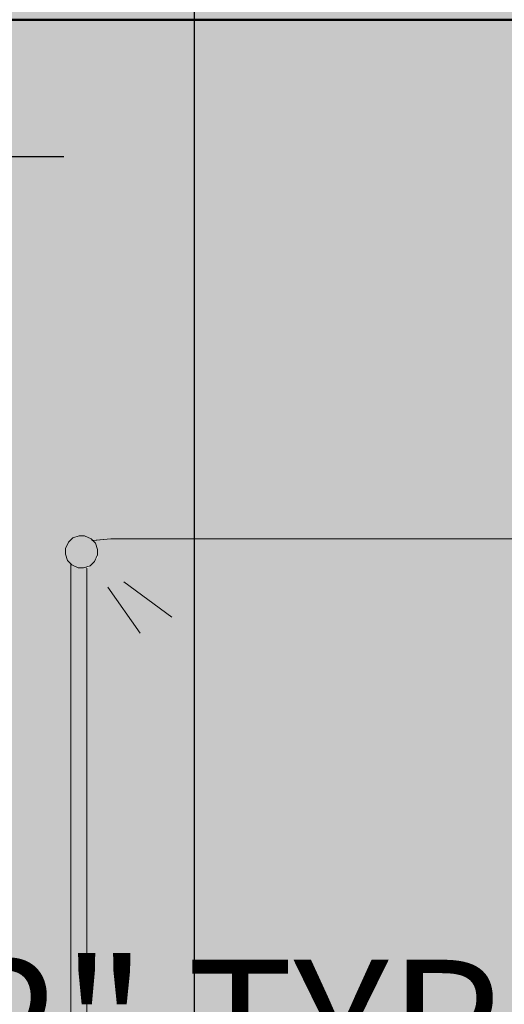
# Model space of a CAD drawing. Units: inches. Extents: x 528 to 2620, y -1066 to 798.
# Tile 29 of 41: x 1157 to 1180, y 665 to 710. Entities that reach past the tile are written whole.
import ezdxf

# ---------------------------------------------------------------- set-up
doc = ezdxf.new("R2010")
doc.units = ezdxf.units.IN
doc.header["$MEASUREMENT"] = 0
for name, color, linetype, lineweight in [('A-ANNO-DIMS', 2, 'Continuous', 18), ('A-FURN', 30, 'Continuous', 18), ('A-WALL', 7, 'Continuous', 50), ('A-WALL-PATT', 8, 'Continuous', 13)]:
    doc.layers.add(name, color=color, linetype=linetype, lineweight=lineweight)
doc.styles.get("Standard").update_dxf_attribs({"font": 'arial.ttf'})
doc.dimstyles.get("Standard").update_dxf_attribs({"dimtxt": 6, "dimasz": 2, "dimexe": 0.18, "dimexo": 0.0625, "dimgap": 0.09, "dimtad": 0, "dimtih": 1, "dimtoh": 1, "dimdec": 1, "dimzin": 0, "dimdsep": 46, "dimlunit": 3, "dimtxsty": 'Standard', "dimblk": 'ARCHTICK', "dimcen": 0.09, "dimadec": 0, "dimazin": 0, "dimtfac": 1, "dimtdec": 1, "dimtofl": 0, "dimtmove": 0, "dimatfit": 3, "dimfxl": 1, "dimtolj": 1, "dimtzin": 0, "dimarcsym": 0})

# ---------------------------------------------------------------- blocks, each defined once
blk = doc.blocks.new('d-bed-3')
at = {"color": 0, "linetype": 'ByBlock'}
for p, q in [((0.7857, -2.0939), (0.7857, -0.0297)), ((0.7857, -0.032), (0.7857, -2.0939)), ((0.8741, -2.0673), (0.9464, -1.9691)), ((0.8851, -2.1005), (0.9795, -2.0342)), ((0.7888, -2.1317), (0.7857, -2.0939)), ((0.7857, -2.0939), (0.7887, -2.1303)), ((0.7948, -2.1259), (0.8078, -2.1215)), ((0.8078, -2.1215), (0.8188, -2.1215)), ((0.8188, -2.1215), (0.8319, -2.1281)), ((0.7797, -2.148), (0.7857, -2.1347)), ((0.7797, -2.148), (0.7857, -2.1347)), ((0.7857, -2.1347), (0.7948, -2.1259)), ((0.7857, -2.1347), (0.7888, -2.1317)), ((0.8319, -2.1281), (0.8409, -2.1369)), ((0.8409, -2.1369), (0.845, -2.1502)), ((2.7264, -2.1436), (0.845, -2.1436)), ((0.7797, -2.159), (0.7797, -2.148)), ((0.7797, -2.148), (0.7797, -2.159)), ((0.7837, -2.1723), (0.7797, -2.159)), ((0.7837, -2.1723), (0.7797, -2.159)), ((0.845, -2.1612), (0.8389, -2.1745)), ((0.845, -2.1502), (0.845, -2.1612)), ((0.7927, -2.1811), (0.7837, -2.1723)), ((0.7927, -2.1811), (0.7837, -2.1723)), ((0.8058, -2.1877), (0.7927, -2.1811)), ((0.8058, -2.1877), (0.7927, -2.1811)), ((0.8299, -2.1833), (0.8168, -2.1877)), ((0.8299, -2.1833), (0.8168, -2.1877)), ((0.8389, -2.1745), (0.8299, -2.1833)), ((0.8367, -2.1767), (0.8299, -2.1833)), ((2.7327, -2.1767), (0.8367, -2.1767)), ((0.8389, -2.1767), (2.7305, -2.1767)), ((0.8168, -2.1877), (0.8058, -2.1877)), ((0.8168, -2.1877), (0.8058, -2.1877))]:
    blk.add_line(p, q, dxfattribs=at)
blk = doc.blocks.new('_ArchTick')
at = {"color": 0, "linetype": 'ByBlock', "const_width": 0.15}
blk.add_lwpolyline([(-0.5, -0.5), (0.5, 0.5)], dxfattribs=at)
blk = doc.blocks.new('*D42')
at = {"layer": 'A-ANNO-DIMS', "color": 0, "lineweight": -2, "transparency": 16777216}
for p, q in [((1159.521, 703.64), (1147.464, 703.64)), ((1147.644, 703.64), (1147.644, 667.032)), ((1147.644, 624.039), (1147.644, 660.647)), ((1159.521, 624.039), (1147.464, 624.039))]:
    blk.add_line(p, q, dxfattribs=at)
at = {"layer": 'Defpoints', "color": 0, "transparency": 16777216}
for p in [(1159.584, 703.64), (1147.644, 624.039), (1159.584, 624.039)]:
    blk.add_point(p, dxfattribs=at)
at = {"layer": 'A-ANNO-DIMS', "color": 0, "lineweight": -2, "transparency": 16777216, "xscale": 2, "yscale": 2, "zscale": 2}
for p, rotation in [((1147.644, 703.64), 90), ((1147.644, 624.039), 270)]:
    blk.add_blockref('_ArchTick', p, dxfattribs=dict(at, rotation=rotation))
at = {"layer": 'A-ANNO-DIMS', "color": 0, "transparency": 16777216, "insert": (1147.644, 663.839), "char_height": 6, "attachment_point": 5}
blk.add_mtext('\\A1;BED 6\'-7 1/2" TYP.', dxfattribs=at)
blk = doc.blocks.new('*D58')
at = {"layer": 'A-ANNO-DIMS', "color": 0, "lineweight": -2, "transparency": 16777216}
for p, q in [((1165.496, 577.985), (1165.496, 751.102)), ((1165.496, 750.922), (1177.395, 750.922)), ((1205.418, 750.922), (1193.52, 750.922)), ((1205.418, 577.985), (1205.418, 751.102))]:
    blk.add_line(p, q, dxfattribs=at)
at = {"layer": 'Defpoints', "color": 0, "transparency": 16777216}
for p in [(1205.418, 750.922), (1165.496, 577.922), (1205.418, 577.922)]:
    blk.add_point(p, dxfattribs=at)
at = {"layer": 'A-ANNO-DIMS', "color": 0, "lineweight": -2, "transparency": 16777216, "xscale": 2, "yscale": 2, "zscale": 2, "rotation": 180}
blk.add_blockref('_ArchTick', (1165.496, 750.922), dxfattribs=at)
at = {"layer": 'A-ANNO-DIMS', "color": 0, "lineweight": -2, "transparency": 16777216, "xscale": 2, "yscale": 2, "zscale": 2}
blk.add_blockref('_ArchTick', (1205.418, 750.922), dxfattribs=at)
at = {"layer": 'A-ANNO-DIMS', "color": 0, "transparency": 16777216, "insert": (1185.457, 750.922), "char_height": 6, "attachment_point": 5}
blk.add_mtext('\\A1;3\'-4"', dxfattribs=at)

msp = doc.modelspace()

# ---------------------------------------------------------------- hatches: boundary and pattern name
at = {"layer": 'A-WALL-PATT', "transparency": 33554521}
h = msp.add_hatch(color=256, dxfattribs=at)
h.dxf.hatch_style = 1
h.paths.add_polyline_path([(1065.996, 709.922), (1114.496, 709.922), (1114.496, 718.922), (1056.996, 718.922), (1056.996, 667.922), (1065.996, 667.922)])
h.paths.add_polyline_path([(1227.496, 718.922), (1162.496, 718.922), (1162.496, 709.922), (1210.996, 709.922), (1210.996, 577.922), (1205.418, 577.922), (1205.496, 573.422), (1210.996, 573.422), (1210.996, 567.422), (1215.496, 567.422), (1215.496, 669.422), (1267.996, 669.422), (1267.996, 675.922), (1263.496, 675.922), (1263.496, 673.922), (1215.496, 673.922), (1215.496, 709.922), (1227.496, 709.922)])
h.paths.add_polyline_path([(1344.996, 718.922), (1315.996, 718.922), (1315.996, 709.922), (1335.996, 709.922), (1335.996, 641.672), (1344.996, 641.672)])
h.paths.add_polyline_path([(1065.996, 619.922), (1056.996, 619.922), (1056.996, 561.422), (1065.996, 561.422), (1065.996, 573.422), (1160.996, 573.422), (1160.996, 569.422), (1165.496, 569.422), (1165.496, 577.922), (1065.996, 577.922)])
h.paths.add_polyline_path([(1215.996, 391.422), (1215.996, 400.422), (1206.996, 400.422), (1200.996, 400.422), (1200.996, 397.422), (1200.996, 391.422), (1206.996, 391.422), (1206.996, 268.922), (1251.996, 268.922), (1251.996, 277.922), (1215.996, 277.922), (1215.996, 359.767)])
h.paths.add_polyline_path([(1344.996, 395.922), (1335.996, 395.922), (1287.996, 395.922), (1287.996, 391.422), (1335.996, 391.422), (1335.996, 277.922), (1299.996, 277.922), (1299.996, 268.922), (1344.996, 268.922)])
h.paths.add_polyline_path([(1344.996, 593.672), (1335.996, 593.672), (1335.996, 525.422), (1215.496, 525.422), (1215.496, 527.172), (1210.996, 527.172), (1210.996, 520.922), (1335.996, 520.922), (1335.996, 443.922), (1344.996, 443.922)])
h.paths.add_polyline_path([(1065.996, 520.922), (1165.496, 520.922), (1165.496, 545.422), (1160.996, 545.422), (1160.996, 525.422), (1065.996, 525.422), (1065.996, 537.422), (1056.996, 537.422), (1056.996, 484.672), (1065.996, 484.672)])
h.paths.add_polyline_path([(1065.996, 436.672), (1056.996, 436.672), (1056.996, 391.422), (1085.496, 391.422), (1085.496, 400.422), (1065.996, 400.422)])
h.paths.add_polyline_path([(1152.996, 397.422), (1152.996, 400.422), (1133.496, 400.422), (1133.496, 391.422), (1152.996, 391.422)])
at = {"layer": 'A-WALL-PATT', "transparency": 33554681}
h = msp.add_hatch(color=256, dxfattribs=at)
h.dxf.hatch_style = 1
h.paths.add_polyline_path([(1061.996, 665.922), (1060.996, 665.922), (1060.996, 621.922), (1061.996, 621.922)])
h.paths.add_polyline_path([(1065.996, 667.922), (1056.996, 667.922), (1056.996, 665.922), (1065.996, 665.922)])
h.paths.add_polyline_path([(1065.996, 621.922), (1056.996, 621.922), (1056.996, 619.922), (1065.996, 619.922)])
h.paths.add_polyline_path([(1160.496, 714.922), (1116.496, 714.922), (1116.496, 713.922), (1160.496, 713.922)])
h.paths.add_polyline_path([(1162.496, 718.922), (1160.496, 718.922), (1160.496, 709.922), (1162.496, 709.922)])
h.paths.add_polyline_path([(1116.496, 718.922), (1114.496, 718.922), (1114.496, 709.922), (1116.496, 709.922)])
h.paths.add_polyline_path([(1251.496, 714.922), (1227.496, 714.922), (1227.496, 713.922), (1251.496, 713.922)])
h.paths.add_polyline_path([(1313.996, 714.922), (1269.996, 714.922), (1269.996, 713.922), (1313.996, 713.922)])
h.paths.add_polyline_path([(1315.996, 718.922), (1313.996, 718.922), (1313.996, 709.922), (1315.996, 709.922)])
h.paths.add_polyline_path([(1269.996, 718.922), (1267.996, 718.922), (1267.996, 709.922), (1269.996, 709.922)])
h.paths.add_polyline_path([(1087.496, 400.422), (1085.496, 400.422), (1085.496, 391.422), (1087.496, 391.422)])
h.paths.add_polyline_path([(1131.496, 396.422), (1087.496, 396.422), (1087.496, 395.422), (1131.496, 395.422)])
h.paths.add_polyline_path([(1133.496, 400.422), (1131.496, 400.422), (1131.496, 391.422), (1133.496, 391.422)])
h.paths.add_polyline_path([(1065.996, 438.672), (1056.996, 438.672), (1056.996, 436.672), (1065.996, 436.672)])
h.paths.add_polyline_path([(1065.996, 484.672), (1056.996, 484.672), (1056.996, 482.672), (1065.996, 482.672)])
h.paths.add_polyline_path([(1061.996, 482.672), (1060.996, 482.672), (1060.996, 438.672), (1061.996, 438.672)])
h = msp.add_hatch(color=256, dxfattribs=at)
h.dxf.hatch_style = 1
h.paths.add_polyline_path([(1065.996, 665.922), (1061.996, 665.922), (1061.996, 621.922), (1065.996, 621.922)])
h.paths.add_polyline_path([(1060.996, 665.922), (1056.996, 665.922), (1056.996, 621.922), (1060.996, 621.922)])
h.paths.add_polyline_path([(1160.496, 713.922), (1116.496, 713.922), (1116.496, 709.922), (1160.496, 709.922)])
h.paths.add_polyline_path([(1160.496, 718.922), (1116.496, 718.922), (1116.496, 714.922), (1160.496, 714.922)])
h.paths.add_polyline_path([(1251.496, 713.922), (1227.496, 713.922), (1227.496, 709.922), (1251.496, 709.922)])
h.paths.add_polyline_path([(1251.496, 718.922), (1227.496, 718.922), (1227.496, 714.922), (1251.496, 714.922)])
h.paths.add_polyline_path([(1313.996, 713.922), (1269.996, 713.922), (1269.996, 709.922), (1313.996, 709.922)])
h.paths.add_polyline_path([(1313.996, 718.922), (1269.996, 718.922), (1269.996, 714.922), (1313.996, 714.922)])
h.paths.add_polyline_path([(1344.996, 639.672), (1340.996, 639.672), (1340.996, 595.672), (1344.996, 595.672)])
h.paths.add_polyline_path([(1339.996, 639.672), (1335.996, 639.672), (1335.996, 595.672), (1339.996, 595.672)])
h.paths.add_polyline_path([(1344.996, 441.922), (1340.996, 441.922), (1340.996, 397.922), (1344.996, 397.922)])
h.paths.add_polyline_path([(1339.996, 441.922), (1335.996, 441.922), (1335.996, 397.922), (1339.996, 397.922)])
h.paths.add_polyline_path([(1297.996, 272.922), (1253.996, 272.922), (1253.996, 268.922), (1297.996, 268.922)])
h.paths.add_polyline_path([(1297.996, 277.922), (1253.996, 277.922), (1253.996, 273.922), (1297.996, 273.922)])
h.paths.add_polyline_path([(1131.496, 395.422), (1087.496, 395.422), (1087.496, 391.422), (1131.496, 391.422)])
h.paths.add_polyline_path([(1131.496, 400.422), (1087.496, 400.422), (1087.496, 396.422), (1131.496, 396.422)])
h.paths.add_polyline_path([(1065.996, 482.672), (1061.996, 482.672), (1061.996, 438.672), (1065.996, 438.672)])
h.paths.add_polyline_path([(1060.996, 482.672), (1056.996, 482.672), (1056.996, 438.672), (1060.996, 438.672)])
h.paths.add_polyline_path([(1065.996, 561.422), (1061.996, 561.422), (1061.996, 537.422), (1065.996, 537.422)])
h.paths.add_polyline_path([(1060.996, 561.422), (1056.996, 561.422), (1056.996, 537.422), (1060.996, 537.422)])
at = {"layer": 'A-WALL-PATT', "transparency": 33554536}
h = msp.add_hatch(color=256, dxfattribs=at)
h.dxf.hatch_style = 1
h.paths.add_polyline_path([(1335.996, 709.922), (1267.996, 709.922), (1267.996, 699.922), (1266.746, 699.922), (1266.746, 675.922), (1267.996, 675.922), (1267.996, 669.422), (1215.496, 669.422), (1215.496, 567.172), (1216.996, 567.172), (1256.996, 567.172), (1256.996, 565.422), (1256.958, 565.422, -0.401453), (1216.996, 527.172), (1215.496, 527.172), (1215.496, 525.422), (1335.996, 525.422)], flags=17)
h.paths.add_polyline_path([(1285.032, 635.927), (1285.229, 636.128), (1285.672, 636.263), (1286.206, 636.02), (1286.976, 636.084), (1332.983, 636.084), (1333.363, 636.222), (1333.82, 636.084), (1334.115, 635.714), (1334.115, 635.3), (1333.907, 634.86), (1333.82, 634.827), (1333.82, 592.738), (1333.967, 592.604), (1334.115, 592.291), (1334.115, 591.877), (1333.82, 591.507), (1333.363, 591.369), (1332.983, 591.507), (1332.638, 591.789), (1332.638, 591.507), (1286.976, 591.507), (1286.173, 591.672), (1286.066, 591.574), (1285.681, 591.37), (1285.229, 591.507), (1285.032, 591.709), (1284.834, 592.098), (1284.983, 592.537), (1285.13, 592.688), (1285.13, 634.948), (1284.983, 635.099), (1284.834, 635.537)], flags=16)
h.paths.add_polyline_path([(1285.032, 635.927), (1285.229, 636.128), (1285.672, 636.263), (1286.206, 636.02), (1286.976, 636.084), (1332.983, 636.084), (1333.363, 636.222), (1333.82, 636.084), (1334.115, 635.714), (1334.115, 635.3), (1333.967, 634.987), (1333.82, 634.853), (1333.82, 592.738), (1333.967, 592.604), (1334.115, 592.291), (1334.115, 591.877), (1333.82, 591.507), (1333.363, 591.369), (1332.983, 591.507), (1332.638, 591.789), (1332.638, 592.246), (1332.638, 635.345), (1332.638, 635.802), (1332.983, 636.084), (1312.232, 636.084), (1311.1, 635.479), (1310.632, 635.479), (1310.435, 635.233), (1309.943, 635.099), (1309.696, 634.987), (1309.056, 634.763), (1308.712, 634.607), (1308.318, 634.607), (1307.752, 634.36), (1307.112, 634.271), (1307.013, 634.114), (1306.767, 634.025), (1307.255, 633.283), (1306.866, 633.04), (1306.767, 632.884), (1306.373, 632.637), (1306.029, 632.548), (1305.536, 632.414), (1315.472, 618.494), (1316.321, 619.388), (1312.773, 622.858), (1319.616, 630.109), (1320.067, 629.676), (1320.109, 629.997), (1320.281, 630.601), (1320.527, 631.183), (1320.527, 632.011), (1320.256, 632.548), (1320.109, 633.13), (1320.06, 633.734), (1320.626, 634.025), (1321.216, 634.159), (1321.856, 634.114), (1322.447, 633.913), (1322.989, 633.622), (1324.096, 633.622), (1324.638, 633.913), (1325.229, 634.07), (1325.869, 634.07), (1326.435, 633.913), (1326.976, 633.622), (1328.355, 633.622), (1328.896, 633.913), (1329.487, 634.114), (1330.103, 634.159), (1330.693, 634.025), (1331.284, 633.734), (1331.235, 633.13), (1331.087, 632.548), (1330.792, 632.011), (1330.792, 631.183), (1331.038, 630.601), (1331.235, 629.997), (1331.284, 629.415), (1331.186, 628.788), (1331.038, 628.184), (1330.792, 627.602), (1330.792, 626.774), (1331.038, 626.193), (1331.235, 625.588), (1331.284, 625.007), (1331.186, 624.38), (1331.038, 623.776), (1330.792, 623.239), (1330.792, 622.366), (1331.038, 621.829), (1331.235, 621.247), (1331.284, 620.598), (1331.186, 619.972), (1331.038, 619.367), (1330.792, 618.83), (1330.792, 617.958), (1331.087, 617.421), (1331.235, 616.884), (1331.284, 616.235), (1331.284, 615.518), (1330.693, 615.272), (1330.103, 615.116), (1329.487, 615.116), (1328.896, 615.317), (1328.355, 615.653), (1326.976, 615.653), (1326.435, 615.317), (1325.869, 615.16), (1325.229, 615.16), (1324.638, 615.317), (1324.096, 615.653), (1323.242, 615.653), (1324.933, 614.042), (1322.978, 611.983), (1324.096, 611.983), (1324.638, 612.274), (1325.278, 612.43), (1325.869, 612.43), (1326.484, 612.274), (1327.026, 611.983), (1328.355, 611.983), (1328.896, 612.274), (1329.487, 612.475), (1330.103, 612.52), (1330.743, 612.386), (1331.284, 612.072), (1331.284, 611.356), (1331.284, 610.752), (1331.087, 610.17), (1330.792, 609.633), (1330.792, 608.805), (1331.087, 608.223), (1331.235, 607.619), (1331.284, 606.993), (1331.235, 606.411), (1331.087, 605.807), (1330.792, 605.225), (1330.792, 604.397), (1331.087, 603.815), (1331.235, 603.211), (1331.284, 602.629), (1331.235, 602.002), (1331.087, 601.398), (1330.792, 600.861), (1330.792, 599.988), (1331.087, 599.451), (1331.235, 598.87), (1331.284, 598.221), (1331.235, 597.594), (1331.087, 596.99), (1330.792, 596.453), (1330.792, 595.58), (1331.087, 595.043), (1331.284, 594.506), (1331.284, 593.857), (1330.743, 593.611), (1330.103, 593.477), (1329.487, 593.477), (1328.896, 593.678), (1328.355, 594.014), (1327.026, 594.014), (1326.484, 593.678), (1325.869, 593.521), (1325.278, 593.521), (1324.638, 593.678), (1324.096, 594.014), (1323.038, 594.014), (1322.496, 593.678), (1321.906, 593.477), (1321.266, 593.477), (1320.626, 593.611), (1320.109, 593.857), (1320.109, 594.506), (1320.281, 595.043), (1320.576, 595.58), (1320.576, 596.453), (1320.281, 596.99), (1320.158, 597.594), (1320.104, 598.015), (1319.616, 597.549), (1315.659, 601.729), (1312.232, 591.574), (1311.74, 591.664), (1311.592, 591.91), (1310.78, 592.402), (1309.549, 592.895), (1308.958, 592.895), (1308.712, 593.029), (1308.564, 593.141), (1307.752, 593.521), (1306.767, 593.611), (1307.248, 594.356), (1306.866, 594.595), (1306.373, 594.842), (1306.029, 595.088), (1305.536, 595.244), (1315.465, 609.354), (1310.927, 613.706), (1315.472, 618.494), (1305.536, 632.414), (1306.029, 632.548), (1306.373, 632.637), (1306.767, 632.884), (1306.866, 633.04), (1307.255, 633.283), (1306.767, 634.025), (1307.013, 634.114), (1307.112, 634.271), (1307.752, 634.36), (1308.318, 634.607), (1308.712, 634.607), (1309.056, 634.763), (1309.696, 634.987), (1309.943, 635.099), (1310.435, 635.233), (1310.632, 635.479), (1311.1, 635.479), (1312.232, 636.084), (1286.976, 636.084), (1286.216, 636.021), (1286.411, 635.444), (1286.213, 635.054), (1286.016, 634.853), (1285.869, 634.808), (1285.869, 592.839), (1286.153, 592.731), (1286.41, 592.188), (1286.231, 591.66), (1286.173, 591.672), (1286.066, 591.574), (1285.681, 591.37), (1285.229, 591.507), (1285.032, 591.709), (1284.834, 592.098), (1284.983, 592.537), (1285.13, 592.688), (1285.13, 634.948), (1284.983, 635.099), (1284.834, 635.537)], flags=0)
h.paths.add_polyline_path([(1322.501, 653.596), (1333.646, 653.596), (1333.646, 637.994), (1322.501, 637.994)], flags=16)
h.paths.add_polyline_path([(1323.616, 652.482), (1332.531, 652.482), (1332.531, 639.108), (1323.616, 639.108)], flags=0)
edge = h.paths.add_edge_path(flags=0)
edge.add_ellipse((1328.073, 645.795), major_axis=(2.245, 2.245), ratio=1, start_angle=405, end_angle=495, ccw=False)
edge.add_ellipse((1328.073, 645.795), major_axis=(2.245, 2.245), ratio=1, start_angle=675, end_angle=765, ccw=False)
edge.add_ellipse((1328.073, 645.795), major_axis=(2.245, 2.245), ratio=1, start_angle=585, end_angle=675, ccw=False)
edge.add_ellipse((1328.073, 645.795), major_axis=(2.245, 2.245), ratio=1, start_angle=495, end_angle=585, ccw=False)
h.paths.add_polyline_path([(1320.576, 628.386), (1320.33, 628.005), (1320.615, 628.548)], flags=0)
h.paths.add_polyline_path([(1317.893, 604.889), (1318.78, 604.643), (1319.764, 604.285), (1318.878, 604.531)], flags=0)
h.paths.add_polyline_path([(1320.33, 599.653), (1320.576, 599.25), (1320.576, 599.16)], flags=0)
h.paths.add_polyline_path([(1322.501, 589.597), (1333.646, 589.597), (1333.646, 573.995), (1322.501, 573.995)], flags=16)
h.paths.add_polyline_path([(1323.616, 588.482), (1332.531, 588.482), (1332.531, 575.109), (1323.616, 575.109)], flags=0)
edge = h.paths.add_edge_path(flags=0)
edge.add_ellipse((1328.073, 581.796), major_axis=(-2.245, 2.245), ratio=1, start_angle=-45, end_angle=45, ccw=False)
edge.add_ellipse((1328.073, 581.796), major_axis=(-2.245, 2.245), ratio=1, start_angle=-135, end_angle=-45, ccw=False)
edge.add_ellipse((1328.073, 581.796), major_axis=(-2.245, 2.245), ratio=1, start_angle=135, end_angle=-135, ccw=False)
edge.add_ellipse((1328.073, 581.796), major_axis=(-2.245, 2.245), ratio=1, start_angle=45, end_angle=135, ccw=False)
h.paths.add_polyline_path([(1264.746, 699.922), (1263.496, 699.922), (1263.496, 709.922), (1215.496, 709.922), (1215.496, 673.922), (1263.496, 673.922), (1263.496, 675.922), (1264.746, 675.922)], flags=16)
h.paths.add_polyline_path([(1162.192, 569.422), (1160.996, 569.422), (1160.996, 573.422), (1065.996, 573.422), (1065.996, 525.422), (1160.996, 525.422), (1160.996, 545.422), (1162.192, 545.422)])
h.paths.add_polyline_path([(1256.958, 565.422), (1256.996, 565.422), (1256.996, 567.172), (1216.996, 567.172), (1215.496, 567.172), (1215.496, 567.422), (1210.996, 567.422), (1210.996, 573.422), (1205.496, 573.422), (1205.418, 577.922), (1210.996, 577.922), (1210.996, 709.922), (1065.996, 709.922), (1065.996, 577.922), (1165.496, 577.922), (1165.496, 569.422), (1164.192, 569.422), (1164.192, 545.422), (1165.496, 545.422), (1165.496, 520.922), (1152.996, 520.922), (1152.996, 484.922), (1101.996, 484.922), (1101.996, 436.422), (1152.996, 436.422), (1152.996, 400.422), (1152.996, 391.422), (1200.996, 391.422), (1200.996, 400.422), (1206.996, 400.422), (1215.996, 400.422), (1215.996, 391.422), (1215.996, 277.922), (1335.996, 277.922), (1335.996, 391.422), (1287.996, 391.422), (1287.996, 395.922), (1335.996, 395.922), (1335.996, 443.922), (1335.996, 520.922), (1210.996, 520.922), (1210.996, 527.172), (1215.496, 527.172), (1216.996, 527.172, 0.401453)])
h.paths.add_polyline_path([(1167.246, 579.422), (1165.496, 579.422), (1165.496, 619.422), (1167.246, 619.422)], flags=16)
h.paths.add_polyline_path([(1227.97, 501.564), (1236.36, 502.031), (1236.36, 492.555), (1227.97, 493.021, -0.254069)], flags=16)
h.paths.add_polyline_path([(1243.336, 515.692, -0.254069), (1251.879, 515.692), (1252.345, 507.301), (1242.87, 507.301)], flags=16)
h.paths.add_polyline_path([(1239.185, 504.685), (1256.03, 504.685), (1256.03, 479.416), (1239.185, 479.416)], flags=16)
h.paths.add_polyline_path([(1227.97, 489.602), (1236.36, 490.068), (1236.36, 480.592), (1227.97, 481.058, -0.254069)], flags=16)
h.paths.add_polyline_path([(1197.201, 624.039), (1197.201, 639.641), (1208.345, 639.641), (1208.345, 624.039)], flags=16)
h.paths.add_polyline_path([(1198.315, 625.153), (1198.315, 638.526), (1207.231, 638.526), (1207.231, 625.153)], flags=0)
h.paths.add_polyline_path([(1258.855, 502.031), (1267.245, 501.564, -0.254069), (1267.245, 493.021), (1258.855, 492.555)], flags=16)
h.paths.add_polyline_path([(1271.589, 519.657), (1333.671, 519.657), (1333.671, 451.595), (1319.087, 451.595), (1319.087, 505.072), (1288.093, 505.072), (1284.447, 505.072, -0.883215), (1270.678, 514.188), (1270.678, 518.745, -0.414214)], flags=16)
h.paths.add_polyline_path([(1331.848, 517.834), (1331.848, 453.418), (1328.202, 453.418), (1328.202, 505.072), (1298.424, 505.072), (1298.424, 514.188), (1288.093, 514.188), (1288.093, 517.834)], flags=0)
h.paths.add_polyline_path([(1242.87, 476.8), (1252.345, 476.8), (1251.879, 468.409, -0.254069), (1243.336, 468.409)], flags=16)
h.paths.add_polyline_path([(1258.855, 490.068), (1267.245, 489.602, -0.254069), (1267.245, 481.058), (1258.855, 480.592)], flags=16)
h.paths.add_polyline_path([(1161.676, 641.551), (1160.873, 641.716), (1160.765, 641.618), (1160.38, 641.414), (1159.928, 641.551), (1159.731, 641.753), (1159.534, 642.142), (1159.682, 642.581), (1159.83, 642.732), (1159.83, 684.992), (1159.682, 685.143), (1159.534, 685.582), (1159.731, 685.971), (1159.928, 686.172), (1160.371, 686.307), (1160.905, 686.064), (1161.676, 686.128), (1207.682, 686.128), (1208.063, 686.266), (1208.519, 686.128), (1208.815, 685.758), (1208.815, 685.344), (1208.607, 684.904), (1208.519, 684.871), (1208.519, 642.782), (1208.667, 642.648), (1208.877, 642.201), (1208.716, 641.797), (1208.519, 641.551), (1208.063, 641.413), (1207.682, 641.551), (1207.338, 641.833), (1207.338, 641.551)], flags=16)
h.paths.add_polyline_path([(1186.931, 641.618), (1186.439, 641.708), (1186.291, 641.954), (1185.479, 642.446), (1184.248, 642.939), (1183.658, 642.939), (1183.411, 643.073), (1183.264, 643.185), (1182.451, 643.565), (1181.467, 643.655), (1181.948, 644.4), (1181.565, 644.639), (1181.073, 644.886), (1180.728, 645.132), (1180.236, 645.288), (1190.164, 659.398), (1185.627, 663.75), (1190.171, 668.538), (1180.236, 682.458), (1180.728, 682.592), (1181.073, 682.681), (1181.467, 682.928), (1181.565, 683.084), (1181.954, 683.327), (1181.467, 684.069), (1181.713, 684.158), (1181.811, 684.315), (1182.451, 684.404), (1183.018, 684.651), (1183.411, 684.651), (1183.756, 684.807), (1184.396, 685.031), (1184.642, 685.143), (1185.135, 685.277), (1185.331, 685.523), (1185.799, 685.523), (1186.931, 686.128), (1161.676, 686.128), (1160.915, 686.065), (1161.111, 685.488), (1160.913, 685.098), (1160.716, 684.897), (1160.568, 684.852), (1160.568, 642.883), (1160.853, 642.775), (1161.109, 642.232), (1160.931, 641.704), (1160.873, 641.716), (1160.765, 641.618), (1160.38, 641.414), (1159.928, 641.551), (1159.731, 641.753), (1159.534, 642.142), (1159.682, 642.581), (1159.83, 642.732), (1159.83, 684.992), (1159.682, 685.143), (1159.534, 685.582), (1159.731, 685.971), (1159.928, 686.172), (1160.371, 686.307), (1160.905, 686.064), (1161.676, 686.128), (1207.682, 686.128), (1208.063, 686.266), (1208.519, 686.128), (1208.815, 685.758), (1208.815, 685.344), (1208.667, 685.031), (1208.519, 684.897), (1208.519, 642.782), (1208.667, 642.648), (1208.877, 642.201), (1208.716, 641.797), (1208.519, 641.551), (1208.063, 641.413), (1207.682, 641.551), (1207.338, 641.833), (1207.338, 642.29), (1207.338, 685.389), (1207.338, 685.846), (1207.682, 686.128), (1186.931, 686.128), (1185.799, 685.523), (1185.331, 685.523), (1185.135, 685.277), (1184.642, 685.143), (1184.396, 685.031), (1183.756, 684.807), (1183.411, 684.651), (1183.018, 684.651), (1182.451, 684.404), (1181.811, 684.315), (1181.713, 684.158), (1181.467, 684.069), (1181.954, 683.327), (1181.565, 683.084), (1181.467, 682.928), (1181.073, 682.681), (1180.728, 682.592), (1180.236, 682.458), (1190.171, 668.538), (1191.021, 669.432), (1187.473, 672.902), (1194.316, 680.153), (1194.767, 679.72), (1194.808, 680.041), (1194.981, 680.645), (1195.227, 681.227), (1195.227, 682.055), (1194.956, 682.592), (1194.808, 683.174), (1194.759, 683.778), (1195.325, 684.069), (1195.916, 684.203), (1196.556, 684.158), (1197.147, 683.957), (1197.688, 683.666), (1198.796, 683.666), (1199.338, 683.957), (1199.928, 684.114), (1200.568, 684.114), (1201.135, 683.957), (1201.676, 683.666), (1203.055, 683.666), (1203.596, 683.957), (1204.187, 684.158), (1204.802, 684.203), (1205.393, 684.069), (1205.984, 683.778), (1205.935, 683.174), (1205.787, 682.592), (1205.491, 682.055), (1205.491, 681.227), (1205.738, 680.645), (1205.935, 680.041), (1205.984, 679.459), (1205.885, 678.832), (1205.738, 678.228), (1205.491, 677.646), (1205.491, 676.818), (1205.738, 676.237), (1205.935, 675.632), (1205.984, 675.051), (1205.885, 674.424), (1205.738, 673.82), (1205.491, 673.283), (1205.491, 672.41), (1205.738, 671.873), (1205.935, 671.291), (1205.984, 670.642), (1205.885, 670.016), (1205.738, 669.411), (1205.491, 668.874), (1205.491, 668.002), (1205.787, 667.465), (1205.935, 666.928), (1205.984, 666.279), (1205.984, 665.563), (1205.393, 665.316), (1204.802, 665.16), (1204.187, 665.16), (1203.596, 665.361), (1203.055, 665.697), (1201.676, 665.697), (1201.135, 665.361), (1200.568, 665.204), (1199.928, 665.204), (1199.338, 665.361), (1198.796, 665.697), (1197.942, 665.697), (1199.633, 664.086), (1197.678, 662.027), (1198.796, 662.027), (1199.338, 662.318), (1199.978, 662.474), (1200.568, 662.474), (1201.184, 662.318), (1201.725, 662.027), (1203.055, 662.027), (1203.596, 662.318), (1204.187, 662.519), (1204.802, 662.564), (1205.442, 662.43), (1205.984, 662.116), (1205.984, 661.4), (1205.984, 660.796), (1205.787, 660.214), (1205.491, 659.677), (1205.491, 658.849), (1205.787, 658.267), (1205.935, 657.663), (1205.984, 657.037), (1205.935, 656.455), (1205.787, 655.851), (1205.491, 655.269), (1205.491, 654.441), (1205.787, 653.859), (1205.935, 653.255), (1205.984, 652.673), (1205.935, 652.046), (1205.787, 651.442), (1205.491, 650.905), (1205.491, 650.032), (1205.787, 649.495), (1205.935, 648.914), (1205.984, 648.265), (1205.935, 647.638), (1205.787, 647.034), (1205.491, 646.497), (1205.491, 645.624), (1205.787, 645.087), (1205.984, 644.55), (1205.984, 643.901), (1205.442, 643.655), (1204.802, 643.521), (1204.187, 643.521), (1203.596, 643.722), (1203.055, 644.058), (1201.725, 644.058), (1201.184, 643.722), (1200.568, 643.565), (1199.978, 643.565), (1199.338, 643.722), (1198.796, 644.058), (1197.738, 644.058), (1197.196, 643.722), (1196.605, 643.521), (1195.965, 643.521), (1195.325, 643.655), (1194.808, 643.901), (1194.808, 644.55), (1194.981, 645.087), (1195.276, 645.624), (1195.276, 646.497), (1194.981, 647.034), (1194.858, 647.638), (1194.803, 648.059), (1194.316, 647.593), (1190.359, 651.773)], flags=16)
h.paths.add_polyline_path([(1195.276, 649.204), (1195.03, 649.697), (1195.276, 649.294)], flags=0)
h.paths.add_polyline_path([(1194.464, 654.329), (1193.578, 654.575), (1192.593, 654.933), (1193.479, 654.687)], flags=0)
h.paths.add_polyline_path([(1195.276, 678.43), (1195.03, 678.049), (1195.314, 678.592)], flags=0)
h.paths.add_polyline_path([(1197.201, 688.038), (1197.201, 703.64), (1208.345, 703.64), (1208.345, 688.038)], flags=16)
h.paths.add_polyline_path([(1198.315, 689.152), (1198.315, 702.526), (1207.231, 702.526), (1207.231, 689.152)], flags=0)
h.paths.add_polyline_path([(1217.099, 329.02), (1230.651, 329.02), (1230.651, 315.468), (1217.099, 315.468)], flags=16)
h.paths.add_polyline_path([(1223.875, 322.244), (1227.263, 322.244), (1227.263, 321.322, -0.414214), (1229.729, 318.856, -1), (1224.797, 318.856), (1223.875, 318.856)], flags=0)
h.paths.add_polyline_path([(1222.115, 325.632, -1), (1218.859, 325.632, -1)], flags=0)
h.paths.add_polyline_path([(1228.25, 325.632, -1), (1226.276, 325.632, -1)], flags=0)
h.paths.add_polyline_path([(1221.533, 318.856, -1), (1219.441, 318.856, -1)], flags=0)
h.paths.add_polyline_path([(1299.145, 293.732), (1299.145, 278.539), (1271.232, 278.539), (1271.232, 293.732)], flags=16)
h.paths.add_polyline_path([(1259.687, 292.213), (1270.624, 292.213, -1), (1270.624, 291.605), (1259.687, 291.605, -1)], flags=16)
h.paths.add_polyline_path([(1259.687, 291.301), (1270.624, 291.301, -1), (1270.624, 290.693), (1259.687, 290.693, -1)], flags=16)
h.paths.add_polyline_path([(1259.687, 290.389), (1270.624, 290.389, -1), (1270.624, 289.782), (1259.687, 289.782, -1)], flags=16)
h.paths.add_polyline_path([(1259.687, 289.478), (1270.624, 289.478, -1), (1270.624, 288.87), (1259.687, 288.87, -1)], flags=16)
h.paths.add_polyline_path([(1259.687, 288.566), (1270.624, 288.566, -1), (1270.624, 287.958), (1259.687, 287.958, -1)], flags=16)
h.paths.add_polyline_path([(1274.406, 292.381), (1283.251, 292.381, -0.414214), (1285.074, 290.558), (1285.074, 283.642, -0.414214), (1283.251, 281.819), (1277.723, 281.819), (1278.673, 280.869, -0.57735), (1279.382, 280.16), (1279.436, 280.106, -1), (1279.027, 279.696), (1278.972, 279.751, -0.57735), (1278.263, 280.46), (1276.904, 281.819), (1274.406, 281.819, -0.414214), (1272.583, 283.642), (1272.583, 290.558, -0.414214)], flags=0)
h.paths.add_polyline_path([(1259.687, 287.655), (1270.624, 287.655, -1), (1270.624, 287.047), (1259.687, 287.047, -1)], flags=16)
h.paths.add_polyline_path([(1259.687, 286.743), (1270.624, 286.743, -1), (1270.624, 286.135), (1259.687, 286.135, -1)], flags=16)
h.paths.add_polyline_path([(1259.687, 285.831), (1270.624, 285.831, -1), (1270.624, 285.224), (1259.687, 285.224, -1)], flags=16)
h.paths.add_polyline_path([(1259.687, 284.92), (1270.624, 284.92, -1), (1270.624, 284.312), (1259.687, 284.312, -1)], flags=16)
h.paths.add_polyline_path([(1259.687, 284.008), (1270.624, 284.008, -1), (1270.624, 283.401), (1259.687, 283.401, -1)], flags=16)
h.paths.add_polyline_path([(1287.823, 292.381), (1296.669, 292.381, -0.414214), (1298.492, 290.558), (1298.492, 283.642, -0.414214), (1296.669, 281.819), (1291.14, 281.819), (1292.09, 280.869, -0.57735), (1292.799, 280.16), (1292.854, 280.106, -1), (1292.445, 279.696), (1292.39, 279.751, -0.57735), (1291.681, 280.46), (1290.322, 281.819), (1287.823, 281.819, -0.414214), (1286, 283.642), (1286, 290.558, -0.414214)], flags=0)
h.paths.add_polyline_path([(1259.687, 283.097), (1270.624, 283.097, -1), (1270.624, 282.489), (1259.687, 282.489, -1)], flags=16)
h.paths.add_polyline_path([(1279.939, 287.607, -1), (1278.01, 287.607, -1)], flags=0)
h.paths.add_polyline_path([(1259.687, 282.185), (1270.624, 282.185, -1), (1270.624, 281.577), (1259.687, 281.577, -1)], flags=16)
h.paths.add_polyline_path([(1259.687, 281.273), (1270.624, 281.273, -1), (1270.624, 280.666), (1259.687, 280.666, -1)], flags=16)
h.paths.add_polyline_path([(1275.156, 284.169, -1), (1274.77, 284.169, -1)], flags=0)
h.paths.add_polyline_path([(1293.357, 287.607, -1), (1291.427, 287.607, -1)], flags=0)
h.paths.add_polyline_path([(1275.144, 280.503), (1276.335, 280.503, -5.828427), (1276.335, 280.117), (1275.144, 280.117, -1)], flags=0)
h.paths.add_polyline_path([(1288.574, 284.169, -1), (1288.188, 284.169, -1)], flags=0)
h.paths.add_polyline_path([(1281.31, 280.503), (1282.501, 280.503, -1), (1282.501, 280.117), (1281.31, 280.117, -5.828427)], flags=0)
h.paths.add_polyline_path([(1288.562, 280.503), (1289.752, 280.503, -5.828427), (1289.752, 280.117), (1288.562, 280.117, -1)], flags=0)
h.paths.add_polyline_path([(1294.727, 280.503), (1295.918, 280.503, -1), (1295.918, 280.117), (1294.727, 280.117, -5.828427)], flags=0)
h.paths.add_polyline_path([(1206.996, 391.422), (1200.996, 391.422), (1061.496, 391.422), (1061.496, 307.96), (1068.996, 307.96), (1068.996, 305.422), (1206.996, 305.422)])
at = {"layer": 'A-WALL-PATT', "transparency": 33554480}
h = msp.add_hatch(color=256, dxfattribs=at)
h.dxf.hatch_style = 1
h.paths.add_polyline_path([(1210.996, 709.922), (1065.996, 709.922), (1065.996, 577.922), (1165.496, 577.922), (1165.496, 579.422), (1165.496, 619.422), (1167.246, 619.422), (1167.246, 619.384, -0.401453), (1205.496, 579.422), (1205.496, 577.922), (1210.996, 577.922)])
h.paths.add_polyline_path([(1160.833, 686.058), (1160.905, 686.064), (1160.765, 686.128)], flags=16)
h.paths.add_polyline_path([(1160.931, 641.704), (1160.931, 641.707), (1160.928, 641.705)], flags=0)
h.paths.add_polyline_path([(1159.83, 684.992), (1159.584, 685.244), (1159.584, 685.82), (1160.016, 686.262), (1160.224, 686.262), (1159.928, 686.172), (1159.731, 685.971), (1159.584, 685.68), (1159.584, 685.434), (1159.682, 685.143), (1159.879, 684.942), (1160.175, 684.807), (1160.421, 684.807), (1160.716, 684.897), (1160.913, 685.098), (1161.111, 685.488), (1161.061, 685.635), (1161.061, 685.249), (1160.568, 684.746), (1160.568, 642.961), (1161.061, 642.514), (1161.061, 641.887), (1160.873, 641.716), (1161.676, 641.551), (1186.533, 641.551), (1186.291, 641.954), (1185.479, 642.446), (1184.248, 642.939), (1183.589, 642.939), (1183.264, 643.185), (1182.451, 643.565), (1181.467, 643.655), (1181.948, 644.4), (1181.565, 644.639), (1181.073, 644.886), (1180.728, 645.132), (1180.236, 645.288), (1190.164, 659.398), (1185.627, 663.75), (1190.171, 668.538), (1180.236, 682.458), (1180.728, 682.592), (1181.073, 682.681), (1181.467, 682.928), (1181.565, 683.084), (1181.954, 683.327), (1181.467, 684.069), (1181.713, 684.158), (1181.811, 684.315), (1182.451, 684.404), (1183.018, 684.651), (1183.411, 684.651), (1183.756, 684.807), (1184.396, 685.031), (1184.642, 685.143), (1185.135, 685.277), (1185.331, 685.523), (1185.799, 685.523), (1186.931, 686.128), (1207.682, 686.128), (1208.063, 686.266), (1208.631, 686.094), (1208.877, 685.478), (1208.607, 684.904), (1208.519, 684.871), (1208.519, 642.782), (1208.815, 642.514), (1208.815, 641.921), (1208.448, 641.462), (1207.792, 641.462), (1207.338, 641.833), (1207.338, 641.551), (1161.676, 641.551), (1160.928, 641.705), (1160.38, 641.414), (1159.816, 641.585), (1159.534, 642.142), (1159.722, 642.699), (1159.83, 642.756)], flags=16)
h.paths.add_polyline_path([(1159.83, 684.992), (1159.584, 685.244), (1159.584, 685.82), (1160.016, 686.262), (1160.224, 686.262), (1159.928, 686.172), (1159.731, 685.971), (1159.584, 685.68), (1159.584, 685.434), (1159.682, 685.143), (1159.83, 684.992), (1159.83, 642.732), (1159.682, 642.581), (1159.584, 642.29), (1159.584, 642.044), (1159.731, 641.753), (1160.016, 641.462), (1160.224, 641.462), (1159.816, 641.585), (1159.534, 642.142), (1159.682, 642.581), (1159.83, 642.732)], flags=0)
h.paths.add_polyline_path([(1207.682, 686.128), (1207.517, 686.128), (1207.488, 686.057)], flags=0)
h.paths.add_polyline_path([(1195.276, 648.712), (1195.287, 648.521), (1195.522, 648.746), (1195.522, 648.802), (1195.276, 649.204)], flags=0)
h.paths.add_polyline_path([(1194.767, 679.72), (1194.808, 680.041), (1194.981, 680.645), (1195.227, 681.227), (1195.227, 682.055), (1194.956, 682.592), (1194.808, 683.174), (1194.759, 683.778), (1195.325, 684.069), (1195.916, 684.203), (1196.556, 684.158), (1197.147, 683.957), (1197.688, 683.666), (1198.796, 683.666), (1199.338, 683.957), (1199.928, 684.114), (1200.568, 684.114), (1201.135, 683.957), (1201.676, 683.666), (1203.055, 683.666), (1203.596, 683.957), (1204.187, 684.158), (1204.802, 684.203), (1205.393, 684.069), (1205.984, 683.778), (1205.935, 683.174), (1205.787, 682.592), (1205.491, 682.055), (1205.491, 681.227), (1205.738, 680.645), (1205.935, 680.041), (1205.984, 679.459), (1205.885, 678.832), (1205.738, 678.228), (1205.491, 677.646), (1205.491, 676.818), (1205.738, 676.237), (1205.935, 675.632), (1205.984, 675.051), (1205.885, 674.424), (1205.738, 673.82), (1205.491, 673.283), (1205.491, 672.41), (1205.738, 671.873), (1205.935, 671.291), (1205.984, 670.642), (1205.885, 670.016), (1205.738, 669.411), (1205.491, 668.874), (1205.491, 668.002), (1205.787, 667.465), (1205.935, 666.928), (1205.984, 666.279), (1205.984, 665.563), (1205.393, 665.316), (1204.802, 665.16), (1204.187, 665.16), (1203.596, 665.361), (1203.055, 665.697), (1201.676, 665.697), (1201.135, 665.361), (1200.568, 665.204), (1199.928, 665.204), (1199.338, 665.361), (1198.796, 665.697), (1197.942, 665.697), (1199.633, 664.086), (1197.678, 662.027), (1198.796, 662.027), (1199.338, 662.318), (1199.978, 662.474), (1200.568, 662.474), (1201.184, 662.318), (1201.725, 662.027), (1203.055, 662.027), (1203.596, 662.318), (1204.187, 662.519), (1204.802, 662.564), (1205.442, 662.43), (1205.984, 662.116), (1205.984, 661.4), (1205.984, 660.796), (1205.787, 660.214), (1205.491, 659.677), (1205.491, 658.849), (1205.787, 658.267), (1205.935, 657.663), (1205.984, 657.037), (1205.935, 656.455), (1205.787, 655.851), (1205.491, 655.269), (1205.491, 654.441), (1205.787, 653.859), (1205.935, 653.255), (1205.984, 652.673), (1205.935, 652.046), (1205.787, 651.442), (1205.491, 650.905), (1205.491, 650.032), (1205.787, 649.495), (1205.935, 648.914), (1205.984, 648.265), (1205.935, 647.638), (1205.787, 647.034), (1205.491, 646.497), (1205.491, 645.624), (1205.787, 645.087), (1205.984, 644.55), (1205.984, 643.901), (1205.442, 643.655), (1204.802, 643.521), (1204.187, 643.521), (1203.596, 643.722), (1203.055, 644.058), (1201.725, 644.058), (1201.184, 643.722), (1200.568, 643.565), (1199.978, 643.565), (1199.338, 643.722), (1198.796, 644.058), (1197.738, 644.058), (1195.522, 644.304), (1205.295, 644.304), (1205.295, 661.445), (1197.125, 661.445), (1199.633, 664.086), (1196.004, 667.543), (1201.479, 673.283), (1195.522, 678.996), (1195.522, 678.922), (1195.31, 678.575), (1195.276, 678.43), (1195.03, 678.049), (1195.276, 678.519), (1195.276, 679.232)], flags=0)
h.paths.add_polyline_path([(1192.593, 654.933), (1193.479, 654.687), (1194.464, 654.329), (1193.578, 654.575)], flags=0)
h.paths.add_polyline_path([(1192.593, 672.79), (1193.43, 673.037), (1194.295, 673.351), (1194.29, 673.358), (1193.578, 673.149)], flags=0)
h.paths.add_polyline_path([(1195.276, 649.294), (1195.03, 649.697), (1195.296, 649.165)], flags=0)
h.paths.add_polyline_path([(1197.201, 639.641), (1208.345, 639.641), (1208.345, 624.039), (1197.201, 624.039)], flags=16)
h.paths.add_polyline_path([(1198.315, 638.526), (1207.231, 638.526), (1207.231, 625.153), (1198.315, 625.153)], flags=0)
edge = h.paths.add_edge_path(flags=0)
edge.add_ellipse((1202.773, 631.84), major_axis=(-2.245, 2.245), ratio=1, start_angle=-45, end_angle=45, ccw=False)
edge.add_ellipse((1202.773, 631.84), major_axis=(-2.245, 2.245), ratio=1, start_angle=-135, end_angle=-45, ccw=False)
edge.add_ellipse((1202.773, 631.84), major_axis=(-2.245, 2.245), ratio=1, start_angle=135, end_angle=-135, ccw=False)
edge.add_ellipse((1202.773, 631.84), major_axis=(-2.245, 2.245), ratio=1, start_angle=45, end_angle=135, ccw=False)
h.paths.add_polyline_path([(1197.201, 688.038), (1197.201, 703.64), (1208.345, 703.64), (1208.345, 688.038)], flags=16)
h.paths.add_polyline_path([(1198.315, 689.152), (1198.315, 702.526), (1207.231, 702.526), (1207.231, 689.152)], flags=0)
edge = h.paths.add_edge_path(flags=0)
edge.add_ellipse((1202.773, 695.839), major_axis=(2.245, 2.245), ratio=1, start_angle=405, end_angle=495, ccw=False)
edge.add_ellipse((1202.773, 695.839), major_axis=(2.245, 2.245), ratio=1, start_angle=675, end_angle=765, ccw=False)
edge.add_ellipse((1202.773, 695.839), major_axis=(2.245, 2.245), ratio=1, start_angle=585, end_angle=675, ccw=False)
edge.add_ellipse((1202.773, 695.839), major_axis=(2.245, 2.245), ratio=1, start_angle=495, end_angle=585, ccw=False)
h.paths.add_polyline_path([(1207.338, 685.389), (1207.338, 685.846), (1207.792, 686.217), (1208.448, 686.217), (1208.815, 685.758), (1208.815, 685.165), (1208.519, 684.897), (1208.519, 642.782), (1208.815, 642.514), (1208.815, 641.921), (1208.448, 641.462), (1207.792, 641.462), (1207.338, 641.833), (1207.338, 642.29)], flags=0)
h.paths.add_polyline_path([(1207.469, 642.678), (1207.989, 643.009), (1208.607, 642.775), (1208.877, 642.201), (1208.631, 641.585), (1208.063, 641.413), (1207.488, 641.622), (1207.284, 642.132)], flags=16)
h.paths.add_polyline_path([(1207.633, 684.897), (1207.879, 684.74), (1208.347, 684.74), (1208.667, 685.031), (1208.815, 685.344), (1208.815, 685.635), (1208.716, 685.881), (1208.448, 686.217), (1208.224, 686.217), (1208.631, 686.094), (1208.877, 685.478), (1208.667, 685.031), (1208.347, 684.74), (1207.786, 684.74)], flags=16)
h.paths.add_polyline_path([(1076.476, 648.31), (1137.071, 648.31), (1137.071, 658.865), (1076.476, 658.865)], flags=24)
h.paths.add_polyline_path([(1076.71, 662.103), (1130.014, 662.103), (1130.014, 672.798), (1076.71, 672.798)], flags=24)

# ---------------------------------------------------------------- linework, layer by layer
at = {"layer": 'A-WALL'}
msp.add_line((1210.996, 709.922), (1065.996, 709.922), dxfattribs=at)

# ---------------------------------------------------------------- block references
at = {"layer": 'A-FURN', "xscale": 22.28859121186505, "yscale": 22.28859121186505, "zscale": 22.28859121186505, "rotation": 270}
msp.add_blockref('d-bed-3', (1208.345, 703.64), dxfattribs=at)

# ---------------------------------------------------------------- dimensions: what is measured, and where the dimension line sits
at = {"layer": 'A-ANNO-DIMS'}
dim = msp.add_linear_dim(base=(1205.418, 750.922), p1=(1165.496, 577.922), p2=(1205.418, 577.922), dimstyle='Standard', override={"dimdec": 1, "dimlfac": 1, "dimrnd": 0, "dimzin": 1, "dimdsep": 46, "dimlunit": 4, "dimfrac": 2}, dxfattribs=at)
dim.commit()
dim.dimension.update_dxf_attribs({"geometry": '*D58', "text_midpoint": (1185.457, 750.922)})
dim = msp.add_linear_dim(base=(1147.644, 624.039), p1=(1159.584, 703.64), p2=(1159.584, 624.039), angle=270, text='BED <> TYP.', dimstyle='Standard', override={"dimdec": 1, "dimrnd": 0, "dimzin": 1, "dimlunit": 4, "dimfrac": 2}, dxfattribs=at)
dim.commit()
dim.dimension.update_dxf_attribs({"geometry": '*D42', "text_midpoint": (1147.644, 663.839)})

doc.saveas('drawing.dxf')
